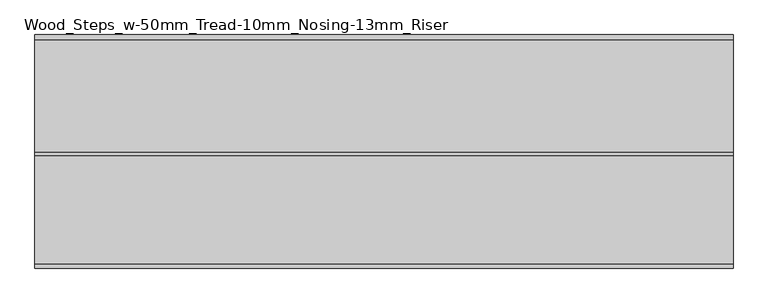
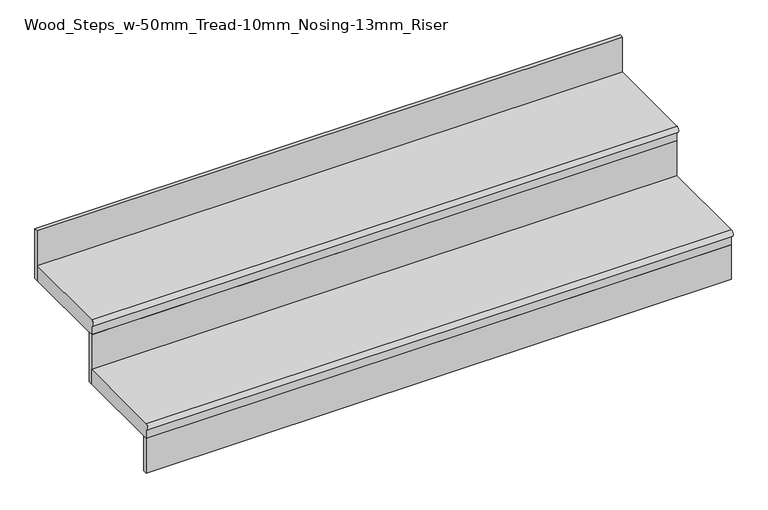
"""IFC4 building model written with IfcOpenShell, lengths in millimetres: stair flight geometry, Wood_Steps_w-50mm_Tread-10mm_Nosing-13mm_Riser."""

from ifc_helpers import new_model, si_unit, point, frame, frame_2d, origin, origin_with_axes, place, context, project, spatial, polyline, circle_curve, trimmed, segment, composite_curve, outline, extrude, source, transform, mapped, element, save


def wood_steps_w_50mm_tread_10mm_nosing_13mm_riser_e56a5079(model_context):
    return source(origin(), model_context, "Body", "SweptSolid", [
        extrude(outline(composite_curve([segment(polyline([(-277.2357414, 166.6666667), (22.7642586, 166.6666667), (22.7642586, 116.6666667), (-277.2357414, 116.6666667), (-277.2357414, 146.6666667)]), True, "CONTINUOUS"), segment(trimmed(circle_curve(frame_2d((-277.2357414, 156.6666667)), 10.0), [point((-277.2357414, 146.6666667))], [point((-277.2357414, 166.6666667))], False, "CARTESIAN"), True, "CONTINUOUS")], self_intersect=False)), frame((-5563.3767794, 0.0, 0.0), z_axis=(1.0, 0.0, 0.0), x_axis=(0.0, 1.0, 0.0)), (0.0, 0.0, 1.0), 1860.0),
        extrude(outline(polyline([(-3703.3767794, -264.7357414), (-3703.3767794, -277.2357414), (-5563.3767794, -277.2357414), (-5563.3767794, -264.7357414), (-3703.3767794, -264.7357414)])), origin_with_axes(), (0.0, 0.0, 1.0), 116.6666667),
        extrude(outline(polyline([(-3703.3767794, 35.2642586), (-3703.3767794, 22.7642586), (-5563.3767794, 22.7642586), (-5563.3767794, 35.2642586), (-3703.3767794, 35.2642586)])), frame((0.0, 0.0, 116.6666667), z_axis=(0.0, 0.0, 1.0), x_axis=(1.0, 0.0, 0.0)), (0.0, 0.0, 1.0), 166.6666667),
        extrude(outline(polyline([(-3703.3767794, 335.2642586), (-3703.3767794, 322.7642586), (-5563.3767794, 322.7642586), (-5563.3767794, 335.2642586), (-3703.3767794, 335.2642586)])), frame((0.0, 0.0, 283.3333333), z_axis=(0.0, 0.0, 1.0), x_axis=(1.0, 0.0, 0.0)), (0.0, 0.0, 1.0), 166.6666667),
        extrude(outline(composite_curve([segment(polyline([(22.7642586, 333.3333333), (322.7642586, 333.3333333), (322.7642586, 283.3333333), (22.7642586, 283.3333333), (22.7642586, 313.3333333)]), True, "CONTINUOUS"), segment(trimmed(circle_curve(frame_2d((22.7642586, 323.3333333)), 10.0), [point((22.7642586, 313.3333333))], [point((22.7642586, 333.3333333))], False, "CARTESIAN"), True, "CONTINUOUS")], self_intersect=False)), frame((-5563.3767794, 0.0, 0.0), z_axis=(1.0, 0.0, 0.0), x_axis=(0.0, 1.0, 0.0)), (0.0, 0.0, 1.0), 1860.0),
    ])


if __name__ == "__main__":
    model = new_model("IFC4")
    model_context = context("Model", 3, world=origin())
    ifc_project = project(units=[si_unit("LENGTHUNIT", "METRE", prefix="MILLI")], contexts=[model_context])
    site = spatial("IfcSite", under=ifc_project)
    building = spatial("IfcBuilding", under=site)
    placement = place(None, origin())
    wood_steps_w_50mm_tread_10mm_nosing_13mm_riser_shape = wood_steps_w_50mm_tread_10mm_nosing_13mm_riser_e56a5079(model_context)
    element("IfcStairFlight", 1, ObjectType="Wood_Steps_w-50mm_Tread-10mm_Nosing-13mm_Riser", at=placement, inside=building, context=model_context, shape_type="MappedRepresentation", body=[
        mapped(wood_steps_w_50mm_tread_10mm_nosing_13mm_riser_shape, transform((0.0, 0.0, 0.0), x_axis=(1.0, 0.0, 0.0), y_axis=(0.0, 1.0, 0.0), z_axis=(0.0, 0.0, 1.0))),
    ])
    save(model, "model.ifc")

# Revit data of these elements
# Element 1 (IfcStairFlight, "Wood_Steps_w-50mm_Tread-10mm_Nosing-13mm_Riser")
#   Materials on its faces: "Oak Flooring"
# Materials
#   "Oak Flooring": class "Wood", colour RGB 212 179 113, transparency 0, Description = "Quercus Rubra", Cost = 0
